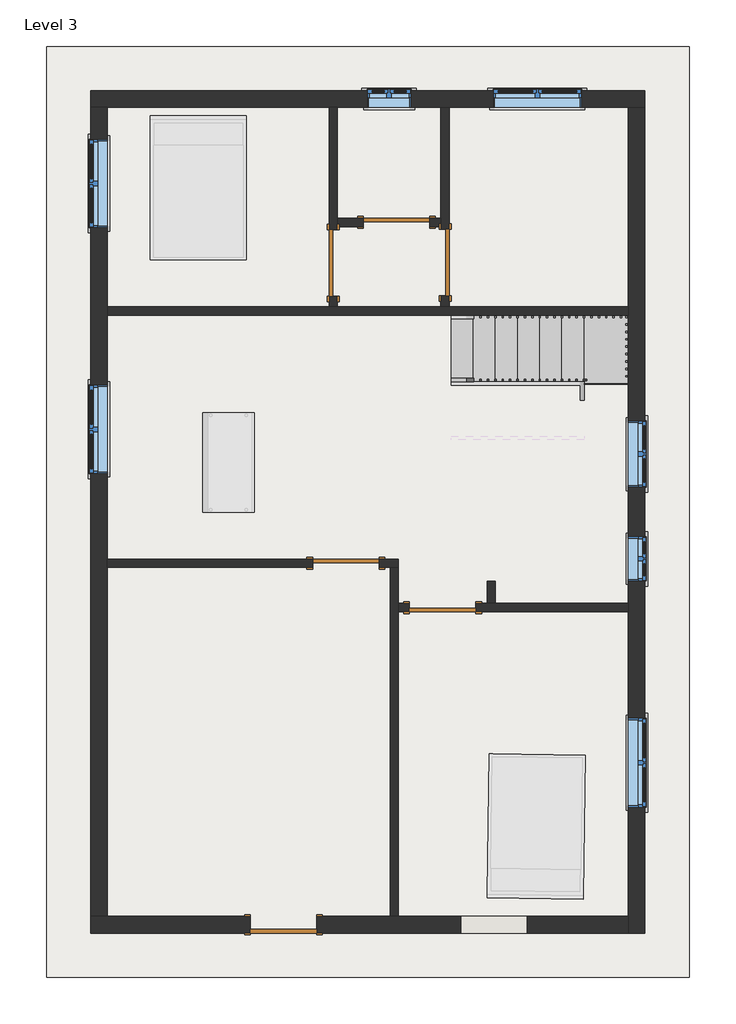
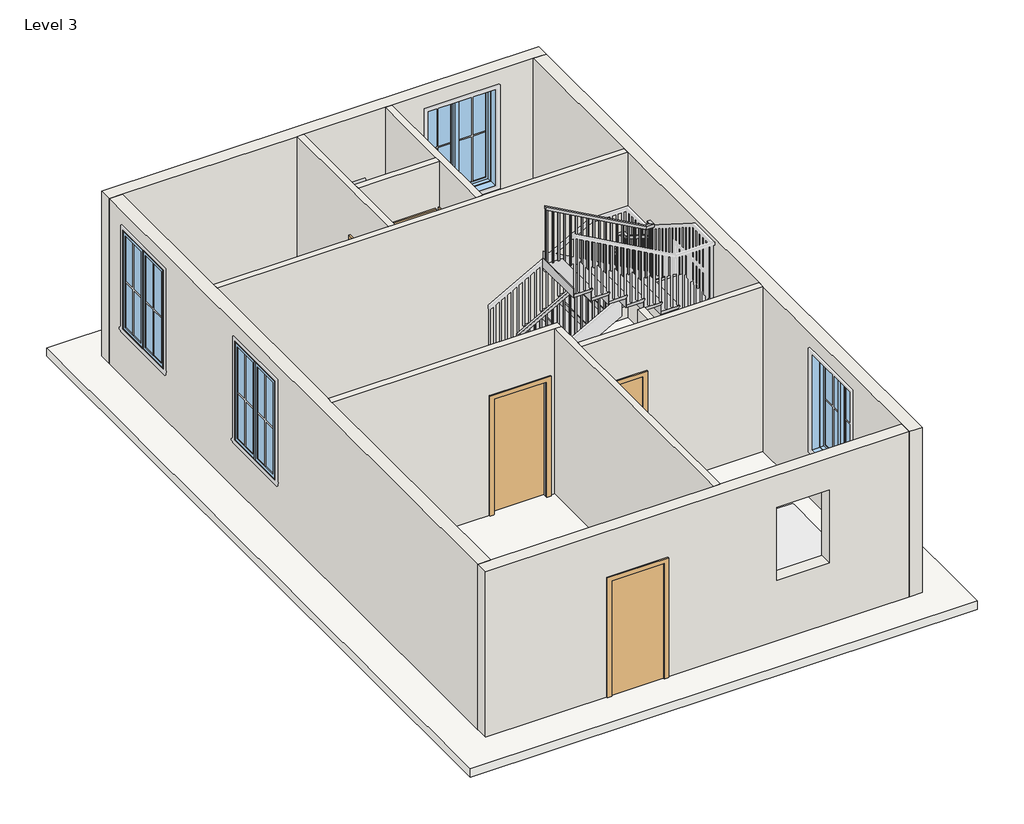
# One storey, part 1 of 2: 12 walls, 7 windows, 6 doors, 1 railing, 1 slab, 1 stair flight.
"""IFC4 building model written with IfcOpenShell, lengths in millimetres."""

from ifc_helpers import new_model, si_unit, frame, origin, place, context, project, spatial, polyline, outline, extrude, faceted_brep, transform, mapped, element, save
from components import door_e5f9f3c4, door_305aa2a5, door_0ca8825f, stair_flight_95d2f6bb, window_c417fced, window_79f73a1a, window_6ca1769e

model = new_model("IFC4")

# Units and contexts
model_context = context("Model", 3, world=origin())
ifc_project = project(units=[si_unit("LENGTHUNIT", "METRE", prefix="MILLI")], contexts=[model_context])

# Site, building, storey
site = spatial("IfcSite", under=ifc_project)
building = spatial("IfcBuilding", under=site)
storey = spatial("IfcBuildingStorey", under=building, Name="Level 3", Elevation=6096.0)

# Doors
placement = place(None, origin())
door_shape = door_e5f9f3c4(model_context)
element("IfcDoor", 1, ObjectType="Single-Flush : 36\" x 84\"", at=placement, inside=storey, context=model_context, shape_type="MappedRepresentation", body=[
    mapped(door_shape, transform((5727.7, 12245.5823212, 6096.0), x_axis=(1.0, 0.0, 0.0), y_axis=(0.0, 1.0, 0.0), z_axis=(0.0, 0.0, 1.0))),
])
element("IfcDoor", 2, ObjectType="Single-Flush : 36\" x 84\"", at=placement, inside=storey, context=model_context, shape_type="MappedRepresentation", body=[
    mapped(door_shape, transform((6394.45, 11693.1323212, 6096.0), x_axis=(0.0, -1.0, 0.0), y_axis=(1.0, 0.0, 0.0), z_axis=(0.0, 0.0, 1.0))),
])
element("IfcDoor", 3, ObjectType="Single-Flush : 36\" x 84\"", at=placement, inside=storey, context=model_context, shape_type="MappedRepresentation", body=[
    mapped(door_shape, transform((6362.7, 6949.6823212, 6096.0), x_axis=(-1.0, 0.0, 0.0), y_axis=(0.0, -1.0, 0.0), z_axis=(0.0, 0.0, 1.0))),
])
element("IfcDoor", 4, ObjectType="Single-Flush : 36\" x 84\"", at=placement, inside=storey, context=model_context, shape_type="MappedRepresentation", body=[
    mapped(door_shape, transform((5029.2, 7559.2823212, 6096.0), x_axis=(1.0, 0.0, 0.0), y_axis=(0.0, 1.0, 0.0), z_axis=(0.0, 0.0, 1.0))),
])
door_2_shape = door_305aa2a5(model_context)
element("IfcDoor", 5, ObjectType="Single-Flush : 36\" x 84\"", at=placement, inside=storey, context=model_context, shape_type="MappedRepresentation", body=[
    mapped(door_2_shape, transform((4857.75, 11689.9573212, 6096.0), x_axis=(0.0, -1.0, 0.0), y_axis=(1.0, 0.0, 0.0), z_axis=(0.0, 0.0, 1.0))),
])
door_3_shape = door_0ca8825f(model_context)
element("IfcDoor", 6, ObjectType="Single-Flush : 36\" x 84\"", at=placement, inside=storey, context=model_context, shape_type="MappedRepresentation", body=[
    mapped(door_3_shape, transform((4171.95, 2587.2323212, 6096.0), x_axis=(-1.0, 0.0, 0.0), y_axis=(0.0, -1.0, 0.0), z_axis=(0.0, 0.0, 1.0))),
])

# Railing
element("IfcRailing", 7, ObjectType="Handrail - Rectangular", at=placement, inside=storey, context=model_context, shape_type="SolidModel", body=[
    faceted_brep([(6477.0, 10105.6323212, 7179.7333333), (6477.0, 10105.6323212, 7121.620221), (6477.0, 10054.8323212, 7121.620221), (6477.0, 10054.8323212, 7179.7333333), (8229.6, 10105.6323212, 8153.4), (8280.4, 10105.6323212, 8123.5091099), (8280.4, 10054.8323212, 8123.5091099), (8229.6, 10054.8323212, 8153.4), (8229.6, 10105.6323212, 8413.447619), (8280.4, 10105.6323212, 8362.647619), (8280.4, 10054.8323212, 8362.647619), (8229.6, 10054.8323212, 8413.447619), (8356.6, 10105.6323212, 8413.447619), (8356.6, 10105.6323212, 8362.647619), (8305.8, 10054.8323212, 8362.647619), (8305.8, 10054.8323212, 8413.447619), (8356.6, 9978.6323212, 8413.447619), (8356.6, 9963.8676405, 8362.647619), (8305.8, 9963.8676405, 8362.647619), (8305.8, 9978.6323212, 8413.447619), (8356.6, 9330.9323212, 8824.6857143), (8356.6, 9280.1323212, 8796.7652821), (8305.8, 9280.1323212, 8796.7652821), (8305.8, 9330.9323212, 8824.6857143), (8356.6, 9330.9323212, 9084.7333333), (8356.6, 9280.1323212, 9033.9333333), (8305.8, 9280.1323212, 9033.9333333), (8305.8, 9330.9323212, 9084.7333333), (8356.6, 9203.9323212, 9084.7333333), (8356.6, 9203.9323212, 9033.9333333), (8305.8, 9254.7323212, 9033.9333333), (8305.8, 9254.7323212, 9084.7333333), (8229.6, 9203.9323212, 9084.7333333), (8216.4363978, 9203.9323212, 9033.9333333), (8216.4363978, 9254.7323212, 9033.9333333), (8229.6, 9254.7323212, 9084.7333333), (6477.0, 9203.9323212, 10058.4), (6477.0, 9254.7323212, 10058.4), (6477.0, 9254.7323212, 10000.2868876), (6477.0, 9203.9323212, 10000.2868876)], [[[0, 1, 2, 3]], [[1, 0, 4, 5]], [[2, 1, 5, 6]], [[3, 2, 6, 7]], [[0, 3, 7, 4]], [[5, 4, 8, 9]], [[6, 5, 9, 10]], [[7, 6, 10, 11]], [[4, 7, 11, 8]], [[9, 8, 12, 13]], [[10, 9, 13, 14]], [[11, 10, 14, 15]], [[8, 11, 15, 12]], [[13, 12, 16, 17]], [[14, 13, 17, 18]], [[15, 14, 18, 19]], [[12, 15, 19, 16]], [[17, 16, 20, 21]], [[18, 17, 21, 22]], [[19, 18, 22, 23]], [[16, 19, 23, 20]], [[21, 20, 24, 25]], [[22, 21, 25, 26]], [[23, 22, 26, 27]], [[20, 23, 27, 24]], [[25, 24, 28, 29]], [[26, 25, 29, 30]], [[27, 26, 30, 31]], [[24, 27, 31, 28]], [[29, 28, 32, 33]], [[30, 29, 33, 34]], [[31, 30, 34, 35]], [[28, 31, 35, 32]], [[36, 37, 38, 39]], [[33, 32, 36, 39]], [[34, 33, 39, 38]], [[35, 34, 38, 37]], [[32, 35, 37, 36]]]),
    extrude(outline(polyline([(9980.8841099, 6511.925), (9991.4674432, 6492.875), (8974.6666667, 6492.875), (8974.6666667, 6511.925), (9980.8841099, 6511.925)])), frame((0.0, 9219.8073212, 0.0), z_axis=(0.0, 1.0, 0.0), x_axis=(0.0, 0.0, 1.0)), (0.0, 0.0, 1.0), 19.05),
    extrude(outline(polyline([(9924.4396654, 6613.525), (9935.0229988, 6594.475), (8974.6666667, 6594.475), (8974.6666667, 6613.525), (9924.4396654, 6613.525)])), frame((0.0, 9219.8073212, 0.0), z_axis=(0.0, 1.0, 0.0), x_axis=(0.0, 0.0, 1.0)), (0.0, 0.0, 1.0), 19.05),
    extrude(outline(polyline([(9867.995221, 6715.125), (9878.5785543, 6696.075), (8974.6666667, 6696.075), (8974.6666667, 6715.125), (9867.995221, 6715.125)])), frame((0.0, 9219.8073212, 0.0), z_axis=(0.0, 1.0, 0.0), x_axis=(0.0, 0.0, 1.0)), (0.0, 0.0, 1.0), 19.05),
    extrude(outline(polyline([(9811.5507765, 6816.725), (9822.1341099, 6797.675), (8805.3333333, 6797.675), (8805.3333333, 6816.725), (9811.5507765, 6816.725)])), frame((0.0, 9219.8073212, 0.0), z_axis=(0.0, 1.0, 0.0), x_axis=(0.0, 0.0, 1.0)), (0.0, 0.0, 1.0), 19.05),
    extrude(outline(polyline([(9755.1063321, 6918.325), (9765.6896654, 6899.275), (8805.3333333, 6899.275), (8805.3333333, 6918.325), (9755.1063321, 6918.325)])), frame((0.0, 9219.8073212, 0.0), z_axis=(0.0, 1.0, 0.0), x_axis=(0.0, 0.0, 1.0)), (0.0, 0.0, 1.0), 19.05),
    extrude(outline(polyline([(9698.6618876, 7019.925), (9709.245221, 7000.875), (8805.3333333, 7000.875), (8805.3333333, 7019.925), (9698.6618876, 7019.925)])), frame((0.0, 9219.8073212, 0.0), z_axis=(0.0, 1.0, 0.0), x_axis=(0.0, 0.0, 1.0)), (0.0, 0.0, 1.0), 19.05),
    extrude(outline(polyline([(9642.2174432, 7121.525), (9652.8007765, 7102.475), (8636.0, 7102.475), (8636.0, 7121.525), (9642.2174432, 7121.525)])), frame((0.0, 9219.8073212, 0.0), z_axis=(0.0, 1.0, 0.0), x_axis=(0.0, 0.0, 1.0)), (0.0, 0.0, 1.0), 19.05),
    extrude(outline(polyline([(9585.7729988, 7223.125), (9596.3563321, 7204.075), (8636.0, 7204.075), (8636.0, 7223.125), (9585.7729988, 7223.125)])), frame((0.0, 9219.8073212, 0.0), z_axis=(0.0, 1.0, 0.0), x_axis=(0.0, 0.0, 1.0)), (0.0, 0.0, 1.0), 19.05),
    extrude(outline(polyline([(9529.3285543, 7324.725), (9539.9118876, 7305.675), (8636.0, 7305.675), (8636.0, 7324.725), (9529.3285543, 7324.725)])), frame((0.0, 9219.8073212, 0.0), z_axis=(0.0, 1.0, 0.0), x_axis=(0.0, 0.0, 1.0)), (0.0, 0.0, 1.0), 19.05),
    extrude(outline(polyline([(9472.8841099, 7426.325), (9483.4674432, 7407.275), (8466.6666667, 7407.275), (8466.6666667, 7426.325), (9472.8841099, 7426.325)])), frame((0.0, 9219.8073212, 0.0), z_axis=(0.0, 1.0, 0.0), x_axis=(0.0, 0.0, 1.0)), (0.0, 0.0, 1.0), 19.05),
    extrude(outline(polyline([(9416.4396654, 7527.925), (9427.0229988, 7508.875), (8466.6666667, 7508.875), (8466.6666667, 7527.925), (9416.4396654, 7527.925)])), frame((0.0, 9219.8073212, 0.0), z_axis=(0.0, 1.0, 0.0), x_axis=(0.0, 0.0, 1.0)), (0.0, 0.0, 1.0), 19.05),
    extrude(outline(polyline([(9359.995221, 7629.525), (9370.5785543, 7610.475), (8466.6666667, 7610.475), (8466.6666667, 7629.525), (9359.995221, 7629.525)])), frame((0.0, 9219.8073212, 0.0), z_axis=(0.0, 1.0, 0.0), x_axis=(0.0, 0.0, 1.0)), (0.0, 0.0, 1.0), 19.05),
    extrude(outline(polyline([(9303.5507765, 7731.125), (9314.1341099, 7712.075), (8297.3333333, 7712.075), (8297.3333333, 7731.125), (9303.5507765, 7731.125)])), frame((0.0, 9219.8073212, 0.0), z_axis=(0.0, 1.0, 0.0), x_axis=(0.0, 0.0, 1.0)), (0.0, 0.0, 1.0), 19.05),
    extrude(outline(polyline([(9247.1063321, 7832.725), (9257.6896654, 7813.675), (8297.3333333, 7813.675), (8297.3333333, 7832.725), (9247.1063321, 7832.725)])), frame((0.0, 9219.8073212, 0.0), z_axis=(0.0, 1.0, 0.0), x_axis=(0.0, 0.0, 1.0)), (0.0, 0.0, 1.0), 19.05),
    extrude(outline(polyline([(9190.6618876, 7934.325), (9201.245221, 7915.275), (8297.3333333, 7915.275), (8297.3333333, 7934.325), (9190.6618876, 7934.325)])), frame((0.0, 9219.8073212, 0.0), z_axis=(0.0, 1.0, 0.0), x_axis=(0.0, 0.0, 1.0)), (0.0, 0.0, 1.0), 19.05),
    extrude(outline(polyline([(9134.2174432, 8035.925), (9144.8007765, 8016.875), (8128.0, 8016.875), (8128.0, 8035.925), (9134.2174432, 8035.925)])), frame((0.0, 9219.8073212, 0.0), z_axis=(0.0, 1.0, 0.0), x_axis=(0.0, 0.0, 1.0)), (0.0, 0.0, 1.0), 19.05),
    extrude(outline(polyline([(9077.7729988, 8137.525), (9088.3563321, 8118.475), (8128.0, 8118.475), (8128.0, 8137.525), (9077.7729988, 8137.525)])), frame((0.0, 9219.8073212, 0.0), z_axis=(0.0, 1.0, 0.0), x_axis=(0.0, 0.0, 1.0)), (0.0, 0.0, 1.0), 19.05),
    extrude(outline(polyline([(9021.3285543, 8239.125), (9031.9118876, 8220.075), (8128.0, 8220.075), (8128.0, 8239.125), (9021.3285543, 8239.125)])), frame((0.0, 9219.8073212, 0.0), z_axis=(0.0, 1.0, 0.0), x_axis=(0.0, 0.0, 1.0)), (0.0, 0.0, 1.0), 19.05),
    extrude(outline(polyline([(8321.675, 9276.9573212), (8340.725, 9276.9573212), (8340.725, 9257.9073212), (8321.675, 9257.9073212), (8321.675, 9276.9573212)])), frame((0.0, 0.0, 7789.3333333), z_axis=(0.0, 0.0, 1.0), x_axis=(1.0, 0.0, 0.0)), (0.0, 0.0, 1.0), 1244.6),
    extrude(outline(polyline([(9359.5073212, 8746.3684567), (9378.5573212, 8734.2732186), (9378.5573212, 7789.3333333), (9359.5073212, 7789.3333333), (9359.5073212, 8746.3684567)])), frame((8321.675, 0.0, 0.0), z_axis=(1.0, 0.0, 0.0), x_axis=(0.0, 1.0, 0.0)), (0.0, 0.0, 1.0), 19.05),
    extrude(outline(polyline([(9461.1073212, 8681.8605202), (9480.1573212, 8669.7652821), (9480.1573212, 7789.3333333), (9461.1073212, 7789.3333333), (9461.1073212, 8681.8605202)])), frame((8321.675, 0.0, 0.0), z_axis=(1.0, 0.0, 0.0), x_axis=(0.0, 1.0, 0.0)), (0.0, 0.0, 1.0), 19.05),
    extrude(outline(polyline([(9562.7073212, 8617.3525837), (9581.7573212, 8605.2573456), (9581.7573212, 7620.0), (9562.7073212, 7620.0), (9562.7073212, 8617.3525837)])), frame((8321.675, 0.0, 0.0), z_axis=(1.0, 0.0, 0.0), x_axis=(0.0, 1.0, 0.0)), (0.0, 0.0, 1.0), 19.05),
    extrude(outline(polyline([(9664.3073212, 8552.8446472), (9683.3573212, 8540.7494091), (9683.3573212, 7620.0), (9664.3073212, 7620.0), (9664.3073212, 8552.8446472)])), frame((8321.675, 0.0, 0.0), z_axis=(1.0, 0.0, 0.0), x_axis=(0.0, 1.0, 0.0)), (0.0, 0.0, 1.0), 19.05),
    extrude(outline(polyline([(9765.9073212, 8488.3367107), (9784.9573212, 8476.2414726), (9784.9573212, 7450.6666667), (9765.9073212, 7450.6666667), (9765.9073212, 8488.3367107)])), frame((8321.675, 0.0, 0.0), z_axis=(1.0, 0.0, 0.0), x_axis=(0.0, 1.0, 0.0)), (0.0, 0.0, 1.0), 19.05),
    extrude(outline(polyline([(9867.5073212, 8423.8287742), (9886.5573212, 8411.7335361), (9886.5573212, 7450.6666667), (9867.5073212, 7450.6666667), (9867.5073212, 8423.8287742)])), frame((8321.675, 0.0, 0.0), z_axis=(1.0, 0.0, 0.0), x_axis=(0.0, 1.0, 0.0)), (0.0, 0.0, 1.0), 19.05),
    extrude(outline(polyline([(9969.1073212, 8359.3208377), (9988.1573212, 8347.2255996), (9988.1573212, 7450.6666667), (9969.1073212, 7450.6666667), (9969.1073212, 8359.3208377)])), frame((8321.675, 0.0, 0.0), z_axis=(1.0, 0.0, 0.0), x_axis=(0.0, 1.0, 0.0)), (0.0, 0.0, 1.0), 19.05),
    extrude(outline(polyline([(8296.275, 10070.7073212), (8296.275, 10089.7573212), (8315.325, 10089.7573212), (8315.325, 10070.7073212), (8296.275, 10070.7073212)])), frame((0.0, 0.0, 7281.3333333), z_axis=(0.0, 0.0, 1.0), x_axis=(1.0, 0.0, 0.0)), (0.0, 0.0, 1.0), 1081.3142857),
    extrude(outline(polyline([(8086.4674432, 8213.725), (8075.8841099, 8194.675), (7112.0, 8194.675), (7112.0, 8213.725), (8086.4674432, 8213.725)])), frame((0.0, 10070.7073212, 0.0), z_axis=(0.0, 1.0, 0.0), x_axis=(0.0, 0.0, 1.0)), (0.0, 0.0, 1.0), 19.05),
    extrude(outline(polyline([(8030.0229988, 8112.125), (8019.4396654, 8093.075), (7112.0, 8093.075), (7112.0, 8112.125), (8030.0229988, 8112.125)])), frame((0.0, 10070.7073212, 0.0), z_axis=(0.0, 1.0, 0.0), x_axis=(0.0, 0.0, 1.0)), (0.0, 0.0, 1.0), 19.05),
    extrude(outline(polyline([(7973.5785543, 8010.525), (7962.995221, 7991.475), (7112.0, 7991.475), (7112.0, 8010.525), (7973.5785543, 8010.525)])), frame((0.0, 10070.7073212, 0.0), z_axis=(0.0, 1.0, 0.0), x_axis=(0.0, 0.0, 1.0)), (0.0, 0.0, 1.0), 19.05),
    extrude(outline(polyline([(7917.1341099, 7908.925), (7906.5507765, 7889.875), (6942.6666667, 7889.875), (6942.6666667, 7908.925), (7917.1341099, 7908.925)])), frame((0.0, 10070.7073212, 0.0), z_axis=(0.0, 1.0, 0.0), x_axis=(0.0, 0.0, 1.0)), (0.0, 0.0, 1.0), 19.05),
    extrude(outline(polyline([(7860.6896654, 7807.325), (7850.1063321, 7788.275), (6942.6666667, 7788.275), (6942.6666667, 7807.325), (7860.6896654, 7807.325)])), frame((0.0, 10070.7073212, 0.0), z_axis=(0.0, 1.0, 0.0), x_axis=(0.0, 0.0, 1.0)), (0.0, 0.0, 1.0), 19.05),
    extrude(outline(polyline([(7804.245221, 7705.725), (7793.6618876, 7686.675), (6942.6666667, 7686.675), (6942.6666667, 7705.725), (7804.245221, 7705.725)])), frame((0.0, 10070.7073212, 0.0), z_axis=(0.0, 1.0, 0.0), x_axis=(0.0, 0.0, 1.0)), (0.0, 0.0, 1.0), 19.05),
    extrude(outline(polyline([(7747.8007765, 7604.125), (7737.2174432, 7585.075), (6773.3333333, 7585.075), (6773.3333333, 7604.125), (7747.8007765, 7604.125)])), frame((0.0, 10070.7073212, 0.0), z_axis=(0.0, 1.0, 0.0), x_axis=(0.0, 0.0, 1.0)), (0.0, 0.0, 1.0), 19.05),
    extrude(outline(polyline([(7691.3563321, 7502.525), (7680.7729988, 7483.475), (6773.3333333, 7483.475), (6773.3333333, 7502.525), (7691.3563321, 7502.525)])), frame((0.0, 10070.7073212, 0.0), z_axis=(0.0, 1.0, 0.0), x_axis=(0.0, 0.0, 1.0)), (0.0, 0.0, 1.0), 19.05),
    extrude(outline(polyline([(7634.9118876, 7400.925), (7624.3285543, 7381.875), (6773.3333333, 7381.875), (6773.3333333, 7400.925), (7634.9118876, 7400.925)])), frame((0.0, 10070.7073212, 0.0), z_axis=(0.0, 1.0, 0.0), x_axis=(0.0, 0.0, 1.0)), (0.0, 0.0, 1.0), 19.05),
    extrude(outline(polyline([(7578.4674432, 7299.325), (7567.8841099, 7280.275), (6604.0, 7280.275), (6604.0, 7299.325), (7578.4674432, 7299.325)])), frame((0.0, 10070.7073212, 0.0), z_axis=(0.0, 1.0, 0.0), x_axis=(0.0, 0.0, 1.0)), (0.0, 0.0, 1.0), 19.05),
    extrude(outline(polyline([(7522.0229988, 7197.725), (7511.4396654, 7178.675), (6604.0, 7178.675), (6604.0, 7197.725), (7522.0229988, 7197.725)])), frame((0.0, 10070.7073212, 0.0), z_axis=(0.0, 1.0, 0.0), x_axis=(0.0, 0.0, 1.0)), (0.0, 0.0, 1.0), 19.05),
    extrude(outline(polyline([(7465.5785543, 7096.125), (7454.995221, 7077.075), (6604.0, 7077.075), (6604.0, 7096.125), (7465.5785543, 7096.125)])), frame((0.0, 10070.7073212, 0.0), z_axis=(0.0, 1.0, 0.0), x_axis=(0.0, 0.0, 1.0)), (0.0, 0.0, 1.0), 19.05),
    extrude(outline(polyline([(7409.1341099, 6994.525), (7398.5507765, 6975.475), (6434.6666667, 6975.475), (6434.6666667, 6994.525), (7409.1341099, 6994.525)])), frame((0.0, 10070.7073212, 0.0), z_axis=(0.0, 1.0, 0.0), x_axis=(0.0, 0.0, 1.0)), (0.0, 0.0, 1.0), 19.05),
    extrude(outline(polyline([(7352.6896654, 6892.925), (7342.1063321, 6873.875), (6434.6666667, 6873.875), (6434.6666667, 6892.925), (7352.6896654, 6892.925)])), frame((0.0, 10070.7073212, 0.0), z_axis=(0.0, 1.0, 0.0), x_axis=(0.0, 0.0, 1.0)), (0.0, 0.0, 1.0), 19.05),
    extrude(outline(polyline([(7296.245221, 6791.325), (7285.6618876, 6772.275), (6434.6666667, 6772.275), (6434.6666667, 6791.325), (7296.245221, 6791.325)])), frame((0.0, 10070.7073212, 0.0), z_axis=(0.0, 1.0, 0.0), x_axis=(0.0, 0.0, 1.0)), (0.0, 0.0, 1.0), 19.05),
    extrude(outline(polyline([(7239.8007765, 6689.725), (7229.2174432, 6670.675), (6265.3333333, 6670.675), (6265.3333333, 6689.725), (7239.8007765, 6689.725)])), frame((0.0, 10070.7073212, 0.0), z_axis=(0.0, 1.0, 0.0), x_axis=(0.0, 0.0, 1.0)), (0.0, 0.0, 1.0), 19.05),
    extrude(outline(polyline([(7183.3563321, 6588.125), (7172.7729988, 6569.075), (6265.3333333, 6569.075), (6265.3333333, 6588.125), (7183.3563321, 6588.125)])), frame((0.0, 10070.7073212, 0.0), z_axis=(0.0, 1.0, 0.0), x_axis=(0.0, 0.0, 1.0)), (0.0, 0.0, 1.0), 19.05),
    extrude(outline(polyline([(8321.675, 9238.8573212), (8340.725, 9238.8573212), (8340.725, 9219.8073212), (8321.675, 9219.8073212), (8321.675, 9238.8573212)])), frame((0.0, 0.0, 7958.6666667), z_axis=(0.0, 0.0, 1.0), x_axis=(1.0, 0.0, 0.0)), (0.0, 0.0, 1.0), 1075.2666667),
    extrude(outline(polyline([(8321.675, 10070.7073212), (8321.675, 10089.7573212), (8340.725, 10089.7573212), (8340.725, 10070.7073212), (8321.675, 10070.7073212)])), frame((0.0, 0.0, 7281.3333333), z_axis=(0.0, 0.0, 1.0), x_axis=(1.0, 0.0, 0.0)), (0.0, 0.0, 1.0), 1081.3142857),
    extrude(outline(polyline([(9989.7035543, 6496.05), (10000.2868876, 6477.0), (8974.6666667, 6477.0), (8974.6666667, 6496.05), (9989.7035543, 6496.05)])), frame((0.0, 9219.8073212, 0.0), z_axis=(0.0, 1.0, 0.0), x_axis=(0.0, 0.0, 1.0)), (0.0, 0.0, 1.0), 19.05),
    extrude(outline(polyline([(7132.2035543, 6496.05), (7121.620221, 6477.0), (6265.3333333, 6477.0), (6265.3333333, 6496.05), (7132.2035543, 6496.05)])), frame((0.0, 10070.7073212, 0.0), z_axis=(0.0, 1.0, 0.0), x_axis=(0.0, 0.0, 1.0)), (0.0, 0.0, 1.0), 19.05),
])

# Slab
element("IfcSlab", 8, ObjectType="Generic - 12\"", at=placement, inside=storey, context=model_context, shape_type="SweptSolid", body=[
    extrude(outline(polyline([(9753.6, 14664.9323212), (9753.6, 1863.3323212), (914.4, 1863.3323212), (914.4, 14664.9323212), (9753.6, 14664.9323212)])), frame((0.0, 0.0, 5943.6), z_axis=(0.0, 0.0, 1.0), x_axis=(1.0, 0.0, 0.0)), (0.0, 0.0, 1.0), 152.4),
])

# Stair flight
stair_flight_shape = stair_flight_95d2f6bb(model_context)
element("IfcStairFlight", 9, ObjectType="2\" Tread 1\" Nosing 1/4\" Riser", at=placement, inside=storey, context=model_context, shape_type="MappedRepresentation", body=[
    mapped(stair_flight_shape, transform((0.0, 0.0, 0.0), x_axis=(1.0, 0.0, 0.0), y_axis=(0.0, 1.0, 0.0), z_axis=(0.0, 0.0, 1.0))),
])

# Walls
element("IfcWall", 10, ObjectType="Generic - 5\"", at=placement, inside=storey, context=model_context, shape_type="Brep", body=[
    faceted_brep([(4800.6, 11232.7573212, 8229.6), (4800.6, 11232.7573212, 6096.0), (4800.6, 11083.5323212, 6096.0), (4800.6, 11083.5323212, 9144.0), (4800.6, 13826.7323212, 9144.0), (4800.6, 13826.7323212, 6096.0), (4800.6, 12147.1573212, 6096.0), (4800.6, 12147.1573212, 8229.6), (4914.9, 11083.5323212, 6096.0), (4914.9, 11232.7573212, 6096.0), (4914.9, 11232.7573212, 8229.6), (4914.9, 12147.1573212, 8229.6), (4914.9, 12147.1573212, 6096.0), (4914.9, 12188.4323212, 6096.0), (4914.9, 12302.7323212, 6096.0), (4914.9, 13826.7323212, 6096.0), (4914.9, 13826.7323212, 9144.0), (4914.9, 12302.7323212, 9144.0), (4914.9, 12188.4323212, 9144.0), (4914.9, 11083.5323212, 9144.0)], [[[0, 1, 2, 3, 4, 5, 6, 7]], [[8, 9, 10, 11, 12, 13, 14, 15, 16, 17, 18, 19]], [[6, 5, 15, 14, 13, 12]], [[2, 1, 9, 8]], [[4, 3, 19, 18, 17, 16]], [[5, 4, 16, 15]], [[3, 2, 8, 19]], [[10, 9, 1, 0]], [[11, 10, 0, 7]], [[12, 11, 7, 6]]]),
])
element("IfcWall", 11, ObjectType="Generic - 5\"", at=placement, inside=storey, context=model_context, shape_type="Brep", body=[
    faceted_brep([(6337.3, 11235.9323212, 8229.6), (6337.3, 11235.9323212, 6096.0), (6337.3, 11083.5323212, 6096.0), (6337.3, 11083.5323212, 9144.0), (6337.3, 12188.4323212, 9144.0), (6337.3, 12302.7323212, 9144.0), (6337.3, 13826.7323212, 9144.0), (6337.3, 13826.7323212, 6096.0), (6337.3, 12302.7323212, 6096.0), (6337.3, 12188.4323212, 6096.0), (6337.3, 12150.3323212, 6096.0), (6337.3, 12150.3323212, 8229.6), (6451.6, 11083.5323212, 6096.0), (6451.6, 11235.9323212, 6096.0), (6451.6, 11235.9323212, 8229.6), (6451.6, 12150.3323212, 8229.6), (6451.6, 12150.3323212, 6096.0), (6451.6, 13826.7323212, 6096.0), (6451.6, 13826.7323212, 9144.0), (6451.6, 11083.5323212, 9144.0)], [[[0, 1, 2, 3, 4, 5, 6, 7, 8, 9, 10, 11]], [[12, 13, 14, 15, 16, 17, 18, 19]], [[2, 1, 13, 12]], [[10, 9, 8, 7, 17, 16]], [[6, 5, 4, 3, 19, 18]], [[7, 6, 18, 17]], [[3, 2, 12, 19]], [[14, 13, 1, 0]], [[15, 14, 0, 11]], [[16, 15, 11, 10]]]),
])
element("IfcWall", 12, ObjectType="Generic - 5\"", at=placement, inside=storey, context=model_context, shape_type="SweptSolid", body=[
    extrude(outline(polyline([(8229.6, 6184.9), (6096.0, 6184.9), (6096.0, 6337.3), (9144.0, 6337.3), (9144.0, 4914.9), (6096.0, 4914.9), (6096.0, 5270.5), (8229.6, 5270.5), (8229.6, 6184.9)])), frame((0.0, 12188.4323212, 0.0), z_axis=(0.0, 1.0, 0.0), x_axis=(0.0, 0.0, 1.0)), (0.0, 0.0, 1.0), 114.3),
])
element("IfcWall", 13, ObjectType="Generic - 5\"", at=placement, inside=storey, context=model_context, shape_type="Brep", body=[
    faceted_brep([(1752.6, 10969.2323212, 6096.0), (8915.4, 10969.2323212, 6096.0), (8915.4, 10969.2323212, 9144.0), (1752.6, 10969.2323212, 9144.0), (1752.6, 11083.5323212, 6096.0), (1752.6, 11083.5323212, 9144.0), (4800.6, 11083.5323212, 9144.0), (4914.9, 11083.5323212, 9144.0), (6337.3, 11083.5323212, 9144.0), (6451.6, 11083.5323212, 9144.0), (8915.4, 11083.5323212, 9144.0), (8915.4, 11083.5323212, 6096.0), (6451.6, 11083.5323212, 6096.0), (6337.3, 11083.5323212, 6096.0), (4914.9, 11083.5323212, 6096.0), (4800.6, 11083.5323212, 6096.0)], [[[0, 1, 2, 3]], [[4, 5, 6, 7, 8, 9, 10, 11, 12, 13, 14, 15]], [[1, 0, 4, 15, 14, 13, 12, 11]], [[3, 2, 10, 9, 8, 7, 6, 5]], [[2, 1, 11, 10]], [[0, 3, 5, 4]]]),
])
element("IfcWall", 14, ObjectType="Generic - 5\"", at=placement, inside=storey, context=model_context, shape_type="Brep", body=[
    faceted_brep([(5486.4, 7502.1323212, 8229.6), (5486.4, 7502.1323212, 6096.0), (5638.8, 7502.1323212, 6096.0), (5753.1, 7502.1323212, 6096.0), (5753.1, 7502.1323212, 9144.0), (5638.8, 7502.1323212, 9144.0), (1752.6, 7502.1323212, 9144.0), (1752.6, 7502.1323212, 6096.0), (4572.0, 7502.1323212, 6096.0), (4572.0, 7502.1323212, 8229.6), (5753.1, 7616.4323212, 6096.0), (5486.4, 7616.4323212, 6096.0), (5486.4, 7616.4323212, 8229.6), (4572.0, 7616.4323212, 8229.6), (4572.0, 7616.4323212, 6096.0), (1752.6, 7616.4323212, 6096.0), (1752.6, 7616.4323212, 9144.0), (5753.1, 7616.4323212, 9144.0)], [[[0, 1, 2, 3, 4, 5, 6, 7, 8, 9]], [[10, 11, 12, 13, 14, 15, 16, 17]], [[8, 7, 15, 14]], [[3, 2, 1, 11, 10]], [[6, 5, 4, 17, 16]], [[7, 6, 16, 15]], [[4, 3, 10, 17]], [[12, 11, 1, 0]], [[13, 12, 0, 9]], [[14, 13, 9, 8]]]),
])
element("IfcWall", 15, ObjectType="Generic - 5\"", at=placement, inside=storey, context=model_context, shape_type="Brep", body=[
    faceted_brep([(5638.8, 7502.1323212, 6096.0), (5638.8, 2701.5323212, 6096.0), (5638.8, 2701.5323212, 9144.0), (5638.8, 7502.1323212, 9144.0), (5753.1, 7502.1323212, 6096.0), (5753.1, 7502.1323212, 9144.0), (5753.1, 7006.8323212, 9144.0), (5753.1, 6892.5323212, 9144.0), (5753.1, 2701.5323212, 9144.0), (5753.1, 2701.5323212, 6096.0), (5753.1, 6892.5323212, 6096.0), (5753.1, 7006.8323212, 6096.0)], [[[0, 1, 2, 3]], [[4, 5, 6, 7, 8, 9, 10, 11]], [[1, 0, 4, 11, 10, 9]], [[3, 2, 8, 7, 6, 5]], [[0, 3, 5, 4]], [[2, 1, 9, 8]]]),
])
element("IfcWall", 16, ObjectType="Generic - 5\"", at=placement, inside=storey, context=model_context, shape_type="Brep", body=[
    faceted_brep([(5905.5, 7006.8323212, 8229.6), (5905.5, 7006.8323212, 6096.0), (5753.1, 7006.8323212, 6096.0), (5753.1, 7006.8323212, 9144.0), (6972.3, 7006.8323212, 9144.0), (7086.6, 7006.8323212, 9144.0), (8915.4, 7006.8323212, 9144.0), (8915.4, 7006.8323212, 6096.0), (7086.6, 7006.8323212, 6096.0), (6972.3, 7006.8323212, 6096.0), (6819.9, 7006.8323212, 6096.0), (6819.9, 7006.8323212, 8229.6), (5753.1, 6892.5323212, 6096.0), (5905.5, 6892.5323212, 6096.0), (5905.5, 6892.5323212, 8229.6), (6819.9, 6892.5323212, 8229.6), (6819.9, 6892.5323212, 6096.0), (8915.4, 6892.5323212, 6096.0), (8915.4, 6892.5323212, 9144.0), (5753.1, 6892.5323212, 9144.0)], [[[0, 1, 2, 3, 4, 5, 6, 7, 8, 9, 10, 11]], [[12, 13, 14, 15, 16, 17, 18, 19]], [[2, 1, 13, 12]], [[10, 9, 8, 7, 17, 16]], [[6, 5, 4, 3, 19, 18]], [[7, 6, 18, 17]], [[3, 2, 12, 19]], [[14, 13, 1, 0]], [[15, 14, 0, 11]], [[16, 15, 11, 10]]]),
])
element("IfcWall", 17, ObjectType="Generic - 5\"", at=placement, inside=storey, context=model_context, shape_type="SweptSolid", body=[
    extrude(outline(polyline([(7086.6, 7311.6323212), (7086.6, 7006.8323212), (6972.3, 7006.8323212), (6972.3, 7311.6323212), (7086.6, 7311.6323212)])), frame((0.0, 0.0, 6096.0), z_axis=(0.0, 0.0, 1.0), x_axis=(1.0, 0.0, 0.0)), (0.0, 0.0, 1.0), 3048.0),
])
element("IfcWall", 18, ObjectType="Generic - 8\"", at=placement, inside=storey, context=model_context, shape_type="Brep", body=[
    faceted_brep([(1524.0, 13826.7323212, 6096.0), (1752.6, 13826.7323212, 6096.0), (4800.6, 13826.7323212, 6096.0), (4914.9, 13826.7323212, 6096.0), (6337.3, 13826.7323212, 6096.0), (6451.6, 13826.7323212, 6096.0), (8915.4, 13826.7323212, 6096.0), (9144.0, 13826.7323212, 6096.0), (9144.0, 13826.7323212, 9144.0), (8915.4, 13826.7323212, 9144.0), (6451.6, 13826.7323212, 9144.0), (6337.3, 13826.7323212, 9144.0), (4914.9, 13826.7323212, 9144.0), (4800.6, 13826.7323212, 9144.0), (1752.6, 13826.7323212, 9144.0), (1524.0, 13826.7323212, 9144.0), (8274.05, 13826.7323212, 8839.2), (8274.05, 13826.7323212, 7010.4), (7054.85, 13826.7323212, 7010.4), (7054.85, 13826.7323212, 8839.2), (5930.9, 13826.7323212, 7924.8), (5930.9, 13826.7323212, 7010.4), (5321.3, 13826.7323212, 7010.4), (5321.3, 13826.7323212, 7924.8), (1524.0, 14055.3323212, 6096.0), (1524.0, 14055.3323212, 9144.0), (9144.0, 14055.3323212, 9144.0), (9144.0, 14055.3323212, 6096.0), (8274.05, 14055.3323212, 8839.2), (7054.85, 14055.3323212, 8839.2), (7054.85, 14055.3323212, 7010.4), (8274.05, 14055.3323212, 7010.4), (5930.9, 14055.3323212, 7924.8), (5321.3, 14055.3323212, 7924.8), (5321.3, 14055.3323212, 7010.4), (5930.9, 14055.3323212, 7010.4)], [[[0, 1, 2, 3, 4, 5, 6, 7, 8, 9, 10, 11, 12, 13, 14, 15], [16, 17, 18, 19], [20, 21, 22, 23]], [[24, 25, 26, 27], [28, 29, 30, 31], [32, 33, 34, 35]], [[7, 6, 5, 4, 3, 2, 1, 0, 24, 27]], [[15, 14, 13, 12, 11, 10, 9, 8, 26, 25]], [[8, 7, 27, 26]], [[0, 15, 25, 24]], [[17, 16, 28, 31]], [[18, 17, 31, 30]], [[19, 18, 30, 29]], [[16, 19, 29, 28]], [[21, 20, 32, 35]], [[22, 21, 35, 34]], [[23, 22, 34, 33]], [[20, 23, 33, 32]]]),
])
element("IfcWall", 19, ObjectType="Generic - 8\"", at=placement, inside=storey, context=model_context, shape_type="Brep", body=[
    faceted_brep([(8915.4, 13826.7323212, 6096.0), (8915.4, 11083.5323212, 6096.0), (8915.4, 10969.2323212, 6096.0), (8915.4, 7006.8323212, 6096.0), (8915.4, 6892.5323212, 6096.0), (8915.4, 2701.5323212, 6096.0), (8915.4, 2472.9323212, 6096.0), (8915.4, 2472.9323212, 9144.0), (8915.4, 2701.5323212, 9144.0), (8915.4, 6892.5323212, 9144.0), (8915.4, 7006.8323212, 9144.0), (8915.4, 10969.2323212, 9144.0), (8915.4, 11083.5323212, 9144.0), (8915.4, 13826.7323212, 9144.0), (8915.4, 4206.4823212, 8839.2), (8915.4, 4206.4823212, 7010.4), (8915.4, 5425.6823212, 7010.4), (8915.4, 5425.6823212, 8839.2), (8915.4, 7315.6010712, 7924.8), (8915.4, 7315.6010712, 7010.4), (8915.4, 7925.2010712, 7010.4), (8915.4, 7925.2010712, 7924.8), (8915.4, 8602.8899384, 8356.6), (8915.4, 8602.8899384, 7010.4), (8915.4, 9517.2899384, 7010.4), (8915.4, 9517.2899384, 8356.6), (9144.0, 13826.7323212, 6096.0), (9144.0, 13826.7323212, 9144.0), (9144.0, 2472.9323212, 9144.0), (9144.0, 2472.9323212, 6096.0), (9144.0, 4206.4823212, 8839.2), (9144.0, 5425.6823212, 8839.2), (9144.0, 5425.6823212, 7010.4), (9144.0, 4206.4823212, 7010.4), (9144.0, 7315.6010712, 7924.8), (9144.0, 7925.2010712, 7924.8), (9144.0, 7925.2010712, 7010.4), (9144.0, 7315.6010712, 7010.4), (9144.0, 8602.8899384, 8356.6), (9144.0, 9517.2899384, 8356.6), (9144.0, 9517.2899384, 7010.4), (9144.0, 8602.8899384, 7010.4)], [[[0, 1, 2, 3, 4, 5, 6, 7, 8, 9, 10, 11, 12, 13], [14, 15, 16, 17], [18, 19, 20, 21], [22, 23, 24, 25]], [[26, 27, 28, 29], [30, 31, 32, 33], [34, 35, 36, 37], [38, 39, 40, 41]], [[6, 5, 4, 3, 2, 1, 0, 26, 29]], [[13, 12, 11, 10, 9, 8, 7, 28, 27]], [[0, 13, 27, 26]], [[7, 6, 29, 28]], [[15, 14, 30, 33]], [[16, 15, 33, 32]], [[17, 16, 32, 31]], [[14, 17, 31, 30]], [[19, 18, 34, 37]], [[20, 19, 37, 36]], [[21, 20, 36, 35]], [[18, 21, 35, 34]], [[23, 22, 38, 41]], [[24, 23, 41, 40]], [[25, 24, 40, 39]], [[22, 25, 39, 38]]]),
])
element("IfcWall", 20, ObjectType="Generic - 8\"", at=placement, inside=storey, context=model_context, shape_type="Brep", body=[
    faceted_brep([(3714.75, 2701.5323212, 8229.6), (3714.75, 2701.5323212, 6096.0), (1752.6, 2701.5323212, 6096.0), (1524.0, 2701.5323212, 6096.0), (1524.0, 2701.5323212, 9144.0), (1752.6, 2701.5323212, 9144.0), (5638.8, 2701.5323212, 9144.0), (5753.1, 2701.5323212, 9144.0), (8915.4, 2701.5323212, 9144.0), (8915.4, 2701.5323212, 6096.0), (5753.1, 2701.5323212, 6096.0), (5638.8, 2701.5323212, 6096.0), (4629.15, 2701.5323212, 6096.0), (4629.15, 2701.5323212, 8229.6), (6610.35, 2701.5323212, 8557.6110953), (6610.35, 2701.5323212, 7211.4110953), (7524.75, 2701.5323212, 7211.4110953), (7524.75, 2701.5323212, 8557.6110953), (1524.0, 2472.9323212, 6096.0), (3714.75, 2472.9323212, 6096.0), (3714.75, 2472.9323212, 8229.6), (4629.15, 2472.9323212, 8229.6), (4629.15, 2472.9323212, 6096.0), (8915.4, 2472.9323212, 6096.0), (8915.4, 2472.9323212, 9144.0), (1524.0, 2472.9323212, 9144.0), (6610.35, 2472.9323212, 8557.6110953), (7524.75, 2472.9323212, 8557.6110953), (7524.75, 2472.9323212, 7211.4110953), (6610.35, 2472.9323212, 7211.4110953)], [[[0, 1, 2, 3, 4, 5, 6, 7, 8, 9, 10, 11, 12, 13], [14, 15, 16, 17]], [[18, 19, 20, 21, 22, 23, 24, 25], [26, 27, 28, 29]], [[3, 2, 1, 19, 18]], [[12, 11, 10, 9, 23, 22]], [[8, 7, 6, 5, 4, 25, 24]], [[9, 8, 24, 23]], [[4, 3, 18, 25]], [[20, 19, 1, 0]], [[21, 20, 0, 13]], [[22, 21, 13, 12]], [[15, 14, 26, 29]], [[16, 15, 29, 28]], [[17, 16, 28, 27]], [[14, 17, 27, 26]]]),
])
element("IfcWall", 21, ObjectType="Generic - 8\"", at=placement, inside=storey, context=model_context, shape_type="Brep", body=[
    faceted_brep([(1752.6, 2701.5323212, 6096.0), (1752.6, 7502.1323212, 6096.0), (1752.6, 7616.4323212, 6096.0), (1752.6, 10969.2323212, 6096.0), (1752.6, 11083.5323212, 6096.0), (1752.6, 13826.7323212, 6096.0), (1752.6, 13826.7323212, 9144.0), (1752.6, 11083.5323212, 9144.0), (1752.6, 10969.2323212, 9144.0), (1752.6, 7616.4323212, 9144.0), (1752.6, 7502.1323212, 9144.0), (1752.6, 2701.5323212, 9144.0), (1752.6, 13390.2194306, 8839.2), (1752.6, 13390.2194306, 7010.4), (1752.6, 12171.0194306, 7010.4), (1752.6, 12171.0194306, 8839.2), (1752.6, 10010.3823212, 8839.2), (1752.6, 10010.3823212, 7010.4), (1752.6, 8791.1823212, 7010.4), (1752.6, 8791.1823212, 8839.2), (1524.0, 2701.5323212, 6096.0), (1524.0, 2701.5323212, 9144.0), (1524.0, 13826.7323212, 9144.0), (1524.0, 13826.7323212, 6096.0), (1524.0, 13390.2194306, 8839.2), (1524.0, 12171.0194306, 8839.2), (1524.0, 12171.0194306, 7010.4), (1524.0, 13390.2194306, 7010.4), (1524.0, 10010.3823212, 8839.2), (1524.0, 8791.1823212, 8839.2), (1524.0, 8791.1823212, 7010.4), (1524.0, 10010.3823212, 7010.4)], [[[0, 1, 2, 3, 4, 5, 6, 7, 8, 9, 10, 11], [12, 13, 14, 15], [16, 17, 18, 19]], [[20, 21, 22, 23], [24, 25, 26, 27], [28, 29, 30, 31]], [[5, 4, 3, 2, 1, 0, 20, 23]], [[11, 10, 9, 8, 7, 6, 22, 21]], [[6, 5, 23, 22]], [[0, 11, 21, 20]], [[13, 12, 24, 27]], [[14, 13, 27, 26]], [[15, 14, 26, 25]], [[12, 15, 25, 24]], [[17, 16, 28, 31]], [[18, 17, 31, 30]], [[19, 18, 30, 29]], [[16, 19, 29, 28]]]),
])

# Windows
window_shape = window_c417fced(model_context)
element("IfcWindow", 22, ObjectType="Window-Casement-Double : 24\" x 36\"", at=placement, inside=storey, context=model_context, shape_type="MappedRepresentation", body=[
    mapped(window_shape, transform((9029.7, 7620.4010712, 6096.0), x_axis=(0.0, -1.0, 0.0), y_axis=(1.0, 0.0, 0.0), z_axis=(0.0, 0.0, 1.0))),
])
element("IfcWindow", 23, ObjectType="Window-Casement-Double : 24\" x 36\"", at=placement, inside=storey, context=model_context, shape_type="MappedRepresentation", body=[
    mapped(window_shape, transform((5626.1, 13941.0323212, 6096.0), x_axis=(1.0, 0.0, 0.0), y_axis=(0.0, 1.0, 0.0), z_axis=(0.0, 0.0, 1.0))),
])
window_2_shape = window_79f73a1a(model_context)
element("IfcWindow", 24, ObjectType="Window-Casement-Double : 36\" x 53\"", at=placement, inside=storey, context=model_context, shape_type="MappedRepresentation", body=[
    mapped(window_2_shape, transform((9029.7, 9060.0899384, 6096.0), x_axis=(0.0, -1.0, 0.0), y_axis=(1.0, 0.0, 0.0), z_axis=(0.0, 0.0, 1.0))),
])
window_3_shape = window_6ca1769e(model_context)
element("IfcWindow", 25, ObjectType="Window-Casement-Double : 48\" x 72\"", at=placement, inside=storey, context=model_context, shape_type="MappedRepresentation", body=[
    mapped(window_3_shape, transform((1638.3, 12780.6194306, 6096.0), x_axis=(0.0, 1.0, 0.0), y_axis=(-1.0, 0.0, 0.0), z_axis=(0.0, 0.0, 1.0))),
])
element("IfcWindow", 26, ObjectType="Window-Casement-Double : 48\" x 72\"", at=placement, inside=storey, context=model_context, shape_type="MappedRepresentation", body=[
    mapped(window_3_shape, transform((7664.45, 13941.0323212, 6096.0), x_axis=(1.0, 0.0, 0.0), y_axis=(0.0, 1.0, 0.0), z_axis=(0.0, 0.0, 1.0))),
])
element("IfcWindow", 27, ObjectType="Window-Casement-Double : 48\" x 72\"", at=placement, inside=storey, context=model_context, shape_type="MappedRepresentation", body=[
    mapped(window_3_shape, transform((9029.7, 4816.0823212, 6096.0), x_axis=(0.0, -1.0, 0.0), y_axis=(1.0, 0.0, 0.0), z_axis=(0.0, 0.0, 1.0))),
])
element("IfcWindow", 28, ObjectType="Window-Casement-Double : 48\" x 72\"", at=placement, inside=storey, context=model_context, shape_type="MappedRepresentation", body=[
    mapped(window_3_shape, transform((1638.3, 9400.7823212, 6096.0), x_axis=(0.0, 1.0, 0.0), y_axis=(-1.0, 0.0, 0.0), z_axis=(0.0, 0.0, 1.0))),
])

save(model, "model.ifc")

# Revit data of these elements
# Type "Single-Flush : 36\" x 84\""
#   Type Mark = "1"
#   Construction Type Id = "MDOOR"
#   Assembly Code = "C1020"
#   Analytic Construction = "Metal"
#   Thickness = 0' - 2"
#   Heat Transfer Coefficient (U) = 0.651978 BTU/(h·ft²·°F)
#   Height = 7' - 0"
#   Trim Projection Ext = 0' - 1"
#   Trim Projection Int = 0' - 1"
#   Trim Width = 0' - 3"
#   Width = 3' - 0"
#   Define Thermal Properties by = 1
#   Define Thermal Properties by = 1
#   Door Material = Door - Panel
#   Frame Material = Door - Frame
#   Visual Light Transmittance = 0
#   Solar Heat Gain Coefficient = 0
#   Function = (empty or 0)
#   Wall Closure = (empty or 0)
# Type "Handrail - Rectangular"
#   Assembly Code = "C2010400"
#   built-in parameter 1008612 = 0.0416667 (stored number, unit not read)
#   built-in parameter 1008611 = 0.0416667 (stored number, unit not read)
#   built-in parameter 1008609 = 0.333333 (stored number, unit not read)
#   built-in parameter 1008604 = 0.166667 (stored number, unit not read)
#   built-in parameter 1008603 = 0.166667 (stored number, unit not read)
#   Railing Height = 3' - 0"
#   built-in parameter 1008630 = 2
#   built-in parameter 1008610 = 2
#   built-in parameter 1008618 = Baluster - Square : 3/4"
# Type "Generic - 12\""
#   Assembly Code = "B1010"
#   Function = 0
#   Layers, outside or top first: 0' - 6" no material (function 1)
# Type "Generic - 5\""
#   Assembly Code = "B2010"
#   Layers, outside or top first: 0' - 4 1/2" no material (function 1)
# Type "Generic - 8\""
#   Assembly Code = "B2010"
#   Layers, outside or top first: 0' - 9" no material (function 1)
# Type "Window-Casement-Double : 24\" x 36\""
#   Type Mark = "14"
#   Fire Rating = "0.5h"
#   Assembly Code = "B2020100"
#   Analytic Construction = "Double glazing - domestic"
#   Frame Extension [instance default] = 0' - 0 1/4"
#   Window Inset [instance default] = 0' - 0"
#   Wall Thickness [instance default] = 0' - 6"
#   Interior Wall Closure [instance default] = 0' - 2 1/4"
#   Half Width = 1' - 0"
#   Visual Light Transmittance = 0.81
#   Thermal Resistance (R) = 1.8146 (h·ft²·°F)/BTU
#   Solar Heat Gain Coefficient = 0.76
#   Rough Width = 2' - 0 1/2"
#   Rough Height = 3' - 0 1/2"
#   Height = 3' - 0"
#   Heat Transfer Coefficient (U) = 0.5511 BTU/(h·ft²·°F)
#   Exterior Wall Closure [instance default] = 0' - 1 1/4"
#   Extension Jamb [instance default] = 0' - 2 1/4"
#   Default Sill Height = 3' - 0"
#   Width = 2' - 0"
#   Define Thermal Properties by = 0
#   Muntin Visibility = yes
#   Interior Trim Visibility [instance default] = yes
#   Exterior Trim Visibility [instance default] = yes
#   Extension Jamb Visibility [instance default] = yes
#   Interior Trim Material = Wood - Stained
#   Muntin Pattern = Muntin Pattern_2x2 : Muntin Pattern_2x2
#   Interior Trim = Trim-Window-Interior-Flat : Picture Frame
#   Interior Frame Material = Wood - Stained
#   Glass Panel Material = Glass
#   Exterior Trim Material = Clad - White
#   Exterior Trim = Trim-Window-Exterior-Flat : with Sill
#   Exterior Frame Material = Clad - White
#   Wall Closure = (empty or 0)
# Type "Window-Casement-Double : 36\" x 53\""
#   Type Mark = "15"
#   Fire Rating = "0.5h"
#   Assembly Code = "B2020100"
#   Analytic Construction = "Double glazing - domestic"
#   Frame Extension [instance default] = 0' - 0 1/4"
#   Window Inset [instance default] = 0' - 0"
#   Wall Thickness [instance default] = 0' - 6"
#   Interior Wall Closure [instance default] = 0' - 2 1/4"
#   Half Width = 1' - 6"
#   Visual Light Transmittance = 0.81
#   Thermal Resistance (R) = 1.8146 (h·ft²·°F)/BTU
#   Solar Heat Gain Coefficient = 0.76
#   Rough Width = 3' - 0 1/2"
#   Rough Height = 4' - 5 1/2"
#   Height = 4' - 5"
#   Heat Transfer Coefficient (U) = 0.5511 BTU/(h·ft²·°F)
#   Exterior Wall Closure [instance default] = 0' - 1 1/4"
#   Extension Jamb [instance default] = 0' - 2 1/4"
#   Default Sill Height = 3' - 0"
#   Width = 3' - 0"
#   Define Thermal Properties by = 0
#   Muntin Visibility = yes
#   Interior Trim Visibility [instance default] = yes
#   Exterior Trim Visibility [instance default] = yes
#   Extension Jamb Visibility [instance default] = yes
#   Interior Trim Material = Wood - Stained
#   Muntin Pattern = Muntin Pattern_2x2 : Muntin Pattern_2x2
#   Interior Trim = Trim-Window-Interior-Flat : Picture Frame
#   Interior Frame Material = Wood - Stained
#   Glass Panel Material = Glass
#   Exterior Trim Material = Clad - White
#   Exterior Trim = Trim-Window-Exterior-Flat : with Sill
#   Exterior Frame Material = Clad - White
#   Wall Closure = (empty or 0)
# Type "Window-Casement-Double : 48\" x 72\""
#   Type Mark = "17"
#   Fire Rating = "0.5h"
#   Assembly Code = "B2020100"
#   Analytic Construction = "Double glazing - domestic"
#   Frame Extension [instance default] = 0' - 0 1/4"
#   Window Inset [instance default] = 0' - 0"
#   Wall Thickness [instance default] = 0' - 6"
#   Interior Wall Closure [instance default] = 0' - 2 1/4"
#   Half Width = 2' - 0"
#   Visual Light Transmittance = 0.81
#   Thermal Resistance (R) = 1.8146 (h·ft²·°F)/BTU
#   Solar Heat Gain Coefficient = 0.76
#   Rough Width = 4' - 0 1/2"
#   Rough Height = 6' - 0 1/2"
#   Height = 6' - 0"
#   Heat Transfer Coefficient (U) = 0.5511 BTU/(h·ft²·°F)
#   Exterior Wall Closure [instance default] = 0' - 1 1/4"
#   Extension Jamb [instance default] = 0' - 2 1/4"
#   Default Sill Height = 3' - 0"
#   Width = 4' - 0"
#   Define Thermal Properties by = 0
#   Muntin Visibility = yes
#   Interior Trim Visibility [instance default] = yes
#   Exterior Trim Visibility [instance default] = yes
#   Extension Jamb Visibility [instance default] = yes
#   Interior Trim Material = Wood - Stained
#   Muntin Pattern = Muntin Pattern_2x2 : Muntin Pattern_2x2
#   Interior Trim = Trim-Window-Interior-Flat : Picture Frame
#   Interior Frame Material = Wood - Stained
#   Glass Panel Material = Glass
#   Exterior Trim Material = Clad - White
#   Exterior Trim = Trim-Window-Exterior-Flat : with Sill
#   Exterior Frame Material = Clad - White
#   Wall Closure = (empty or 0)
# Elements 1, 2, 3, 4, 5, 6 (IfcDoor, "Single-Flush : 36\" x 84\"")
#   Phase Created = New Construction
#   Materials on its faces: "Door - Frame", "Door - Panel"
# Element 7 (IfcRailing, "Handrail - Rectangular")
#   Phase Created = New Construction
# Element 8 (IfcSlab, "Generic - 12\"")
#   Height Offset From Level = 0' - 0"
#   Phase Created = New Construction
#   Materials on its faces: "Carpet (1)", "Default Floor"
# Element 9 (IfcStairFlight, "2\" Tread 1\" Nosing 1/4\" Riser")
#   Phase Created = New Construction
# Elements 10, 11, 12, 13, 14, 15, 16, 17 (IfcWall, "Generic - 5\"")
#   Top Offset = 0' - 0"
#   Base Offset = 0' - 0"
#   wall height = 10' - 0"
#   Phase Created = New Construction
#   Base Constraint = Level 3
#   Top Constraint = Level 4
#   Materials on its faces: "Default Wall"
# Elements 18, 19, 20, 21 (IfcWall, "Generic - 8\"")
#   Top Offset = 0' - 0"
#   Base Offset = 0' - 0"
#   Unconnected Height = 10' - 0"
#   wall height = 10' - 0"
#   Phase Created = New Construction
#   Base Constraint = Level 3
#   Materials on its faces: "Default Wall", "Wood - Stained"
# Element 22 (IfcWindow, "Window-Casement-Double : 24\" x 36\"")
#   Mark = "19"
#   Window Inset = 0' - 0"
#   Interior Wall Closure = 0' - 2 1/4"
#   Frame Extension = 0' - 0 1/4"
#   Exterior Wall Closure = 0' - 1 1/4"
#   Interior Trim Visibility = yes
#   Exterior Trim Visibility = yes
#   Phase Created = New Construction
#   Materials on its faces: "Wood - Stained", "Glass", "Clad - White"
# Element 23 (IfcWindow, "Window-Casement-Double : 24\" x 36\"")
#   Mark = "20"
#   Window Inset = 0' - 0"
#   Interior Wall Closure = 0' - 2 1/4"
#   Frame Extension = 0' - 0 1/4"
#   Exterior Wall Closure = 0' - 1 1/4"
#   Interior Trim Visibility = yes
#   Exterior Trim Visibility = yes
#   Phase Created = New Construction
#   Materials on its faces: "Wood - Stained", "Glass", "Clad - White"
# Element 24 (IfcWindow, "Window-Casement-Double : 36\" x 53\"")
#   Mark = "21"
#   Window Inset = 0' - 0"
#   Interior Wall Closure = 0' - 2 1/4"
#   Frame Extension = 0' - 0 1/4"
#   Exterior Wall Closure = 0' - 1 1/4"
#   Interior Trim Visibility = yes
#   Exterior Trim Visibility = yes
#   Phase Created = New Construction
#   Materials on its faces: "Wood - Stained", "Glass", "Clad - White"
# Element 25 (IfcWindow, "Window-Casement-Double : 48\" x 72\"")
#   Mark = "15"
#   Window Inset = 0' - 0"
#   Interior Wall Closure = 0' - 2 1/4"
#   Frame Extension = 0' - 0 1/4"
#   Exterior Wall Closure = 0' - 1 1/4"
#   Interior Trim Visibility = yes
#   Exterior Trim Visibility = yes
#   Phase Created = New Construction
#   Materials on its faces: "Wood - Stained", "Glass", "Clad - White"
# Element 26 (IfcWindow, "Window-Casement-Double : 48\" x 72\"")
#   Mark = "16"
#   Window Inset = 0' - 0"
#   Interior Wall Closure = 0' - 2 1/4"
#   Frame Extension = 0' - 0 1/4"
#   Exterior Wall Closure = 0' - 1 1/4"
#   Interior Trim Visibility = yes
#   Exterior Trim Visibility = yes
#   Phase Created = New Construction
#   Materials on its faces: "Wood - Stained", "Glass", "Clad - White"
# Element 27 (IfcWindow, "Window-Casement-Double : 48\" x 72\"")
#   Mark = "17"
#   Window Inset = 0' - 0"
#   Interior Wall Closure = 0' - 2 1/4"
#   Frame Extension = 0' - 0 1/4"
#   Exterior Wall Closure = 0' - 1 1/4"
#   Interior Trim Visibility = yes
#   Exterior Trim Visibility = yes
#   Phase Created = New Construction
#   Materials on its faces: "Wood - Stained", "Glass", "Clad - White"
# Element 28 (IfcWindow, "Window-Casement-Double : 48\" x 72\"")
#   Mark = "18"
#   Window Inset = 0' - 0"
#   Interior Wall Closure = 0' - 2 1/4"
#   Frame Extension = 0' - 0 1/4"
#   Exterior Wall Closure = 0' - 1 1/4"
#   Interior Trim Visibility = yes
#   Exterior Trim Visibility = yes
#   Phase Created = New Construction
#   Materials on its faces: "Wood - Stained", "Glass", "Clad - White"
# Materials
#   "Door - Panel": class "Wood", colour RGB 210 159 95, transparency 0, Cost = 0
#   "Door - Frame": colour RGB 118 70 51, transparency 0, Cost = 0
#   "Wood - Stained": class "Wood", colour RGB 224 178 126, transparency 0, Cost = 0
#   "Glass": class "Glass", colour RGB 0 128 192, transparency 0.75, Description = "Soda Lime Glass", Cost = 0
#   "Clad - White": class "Wood", colour RGB 242 242 238, transparency 0, Cost = 0
#   "Carpet (1)": class "Carpet", colour RGB 124 80 67, transparency 0, Description = "Interior finish", Cost = 0
#   "Default Floor": colour RGB 128 128 128, transparency 0, Cost = 0
#   "Default Wall": colour RGB 128 128 128, transparency 0, Cost = 0
